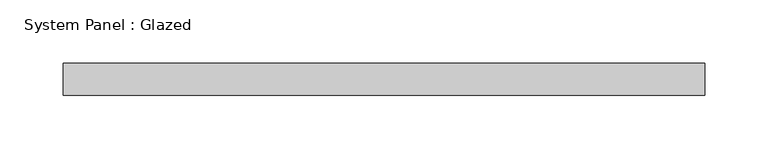
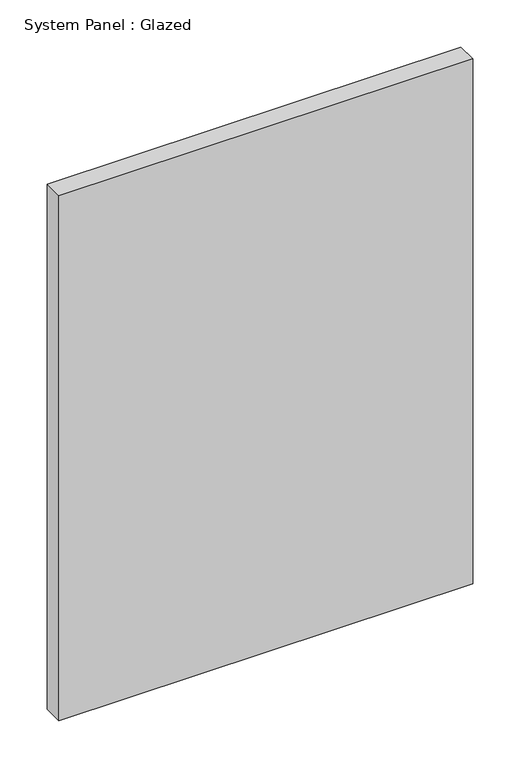
"""IFC4 building model written with IfcOpenShell, lengths in millimetres: plate geometry, System Panel : Glazed."""

from ifc_helpers import new_model, si_unit, origin, origin_with_axes, place, context, project, spatial, polyline, outline, extrude, source, transform, mapped, element, save


def system_panel_glazed_3f6201ba(model_context):
    return source(origin(), model_context, "Body", "SweptSolid", [
        extrude(outline(polyline([(254.0, 19.05), (-254.0, 19.05), (-254.0, 44.45), (254.0, 44.45), (254.0, 19.05)])), origin_with_axes(), (0.0, 0.0, 1.0), 681.3532277),
    ])


if __name__ == "__main__":
    model = new_model("IFC4")
    model_context = context("Model", 3, world=origin())
    ifc_project = project(units=[si_unit("LENGTHUNIT", "METRE", prefix="MILLI")], contexts=[model_context])
    site = spatial("IfcSite", under=ifc_project)
    building = spatial("IfcBuilding", under=site)
    placement = place(None, origin())
    system_panel_glazed_shape = system_panel_glazed_3f6201ba(model_context)
    element("IfcPlate", 1, ObjectType="System Panel : Glazed", at=placement, inside=building, context=model_context, shape_type="MappedRepresentation", body=[
        mapped(system_panel_glazed_shape, transform((0.0, 0.0, 0.0), x_axis=(1.0, 0.0, 0.0), y_axis=(0.0, 1.0, 0.0), z_axis=(0.0, 0.0, 1.0))),
    ])
    save(model, "model.ifc")

# Revit data of these elements
# Type "System Panel : Glazed"
#   Construction Type Id = "GSP4R"
#   Analytic Construction = "1/8 in Pilkington single glazing"
#   Visual Light Transmittance = 0.9
#   Solar Heat Gain Coefficient = 0.86
#   Heat Transfer Coefficient (U) = 1.18115 BTU/(h·ft²·°F)
#   Define Thermal Properties by = 1
# Element 1 (IfcPlate, "System Panel : Glazed")
#   Materials on its faces: "Glass"
# Materials
#   "Glass": class "Glass", colour RGB 0 128 192, transparency 0.75, Description = "Soda Lime Glass", Cost = 0
